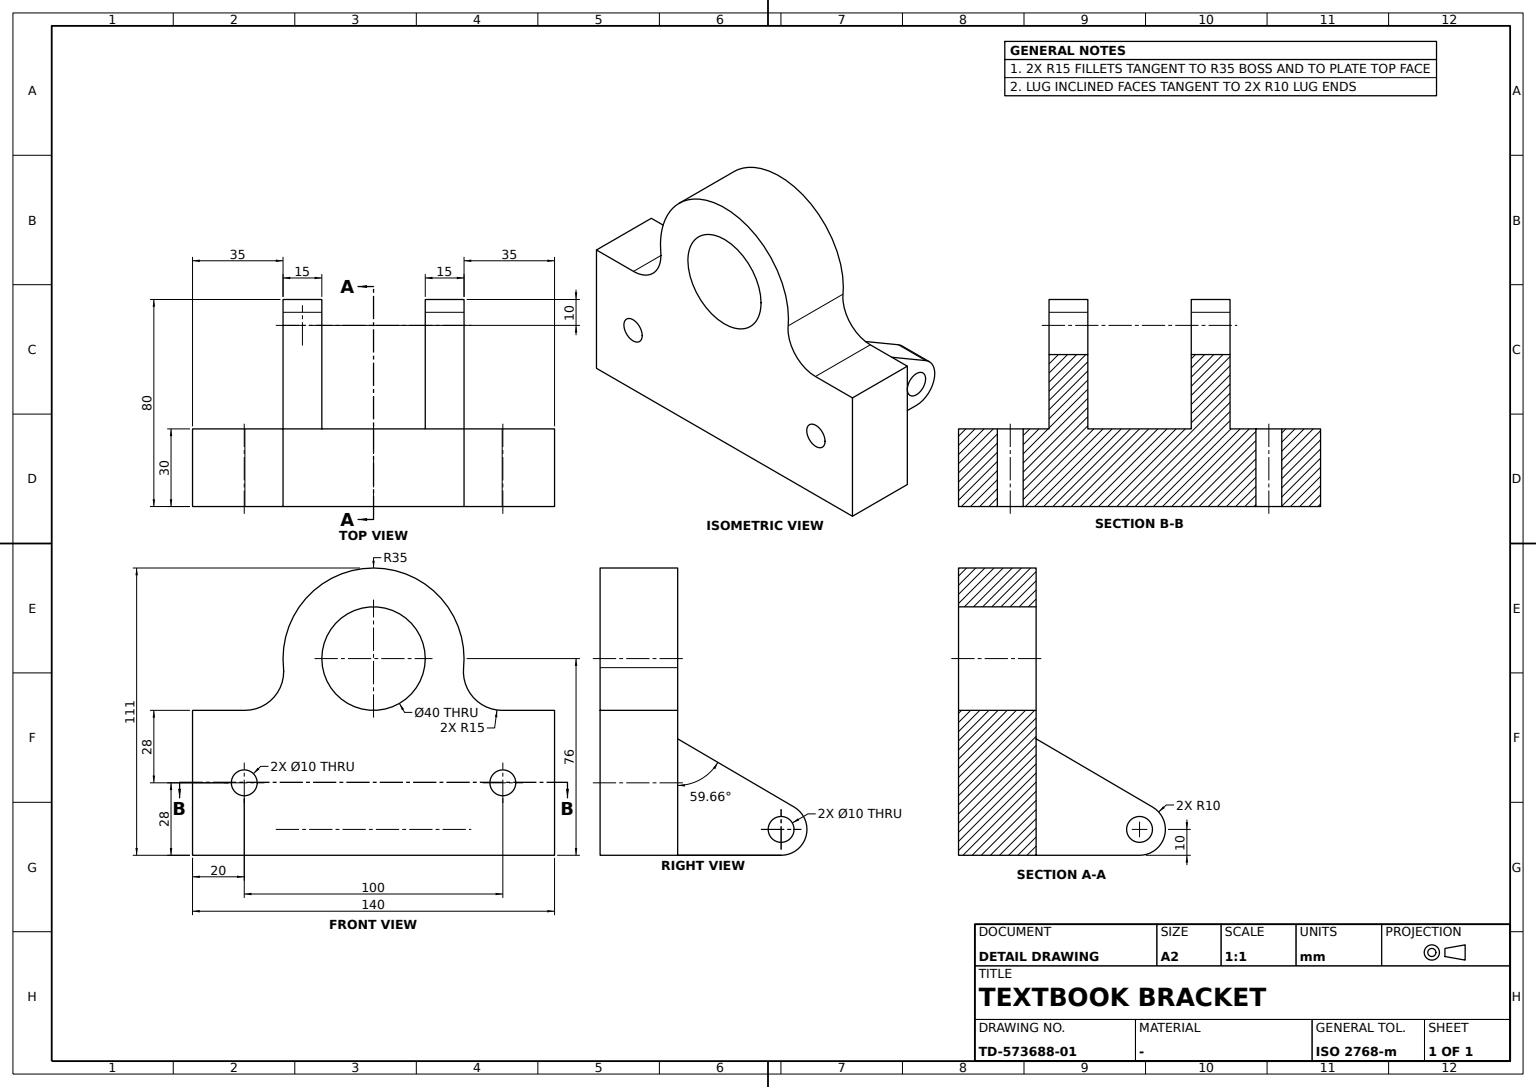
CATIA V5 part; units mm, degrees
sketch "Sketch1" plane through (0, 0, 0) normal (1, 0, 0) x (0, 1, 0)
  line L0 (-70, 0) -> (70, 0)
  line L1 (70, 0) -> (70, 56)
  line L2 (-70, 0) -> (-70, 56)
  point P0 (0, 76)
  arc A0 (34.8246, 72.5) -> (-34.8246, 72.5) centre (0, 76) ccw
  line L3 (-70, 56) -> (-49.7494, 56)
  line L4 (70, 56) -> (49.7494, 56)
  arc A1 (-34.8246, 72.5) -> (-49.7494, 56) centre (-49.7494, 71) cw
  arc A2 (34.8246, 72.5) -> (49.7494, 56) centre (49.7494, 71) ccw
  dimension "length L0" = 140
  dimension "length L1" = 56
  dimension "length L2" = 56
  dimension "distance P0 L0" = 76
  dimension "radius A0" = 35
  dimension "radius A1" = 15
  dimension "radius A2" = 15
  constraint midpoint L0 origin
  constraint horizontal L0 x-axis
  constraint horizontal L3 x-axis
  constraint horizontal L4 x-axis
  constraint vertical L1 y-axis
  constraint vertical L2 y-axis
  constraint coincidence P0 y-axis
  constraint tangency A1 L3
  constraint tangency A1 A0
  constraint tangency A2 A0
  constraint tangency A2 L4
extrude "Pad1" add sketch "Sketch1" along normal blind 30
sketch "Sketch2" plane through (30, 0, 0) normal (1, 0, 0) x (0, 1, 0)
  circle A0 centre (0, 76) radius 20
  arc A1 (34.8246, 72.5) -> (-34.8246, 72.5) centre (0, 76) ccw construction
  dimension "radius A0" = 20
  constraint concentricity A0 A1
extrude "Pocket1" cut sketch "Sketch2" against normal blind 30
sketch "Sketch3" plane through (30, 0, 0) normal (1, 0, 0) x (0, 1, 0)
  circle A0 centre (50, 28) radius 5
  point P0 (50, 28)
  line L0 (-70, 0) -> (70, 0) construction
  circle A1 centre (-50, 28) radius 5
  point P1 (-50, 28)
  dimension "distance P0 L0" = 28
  dimension "distance P0 y axis" = 50
  dimension "radius A0" = 5
  dimension "distance P1 L0" = 28
  dimension "distance P1 y axis" = 50
  dimension "radius A1" = 5
extrude "Pocket2" cut sketch "Sketch3" against normal blind 30
sketch "Sketch4" plane through (0, 0, 0) normal (0, 1, 0) x (-1, 0, 0)
  line L0 (0, 0) -> (40, 0)
  arc A0 (40, 0) -> (45.0515, 18.6303) centre (40, 10) ccw
  line L1 (0, 45) -> (45.0515, 18.6303)
  point P0 (0, 45)
  line L2 (0, 45) -> (0, 0)
  dimension "length L0" = 40
  dimension "radius A0" = 10
  dimension "distance P0 L0" = 45
  constraint horizontal L0 x-axis
  constraint tangency A0 L0
  constraint tangency L1 A0
  constraint coincidence P0 y-axis
  constraint vertical L2 y-axis
extrude "Pad2" add sketch "Sketch4" along normal blind 15 from surface at 20
mirror "Mirror1" about plane through (0, 0, 0) normal (0, 1, 0) of "Pad2"
sketch "Sketch5" plane through (0, 0, 0) normal (0, 1, 0) x (-1, 0, 0)
  circle A0 centre (40, 10) radius 5
  arc A1 (40, 0) -> (45.0515, 18.6303) centre (40, 10) ccw construction
  dimension "radius A0" = 5
  constraint concentricity A0 A1
extrude "Pocket3" cut sketch "Sketch5" against normal through all and the other way blind 35
